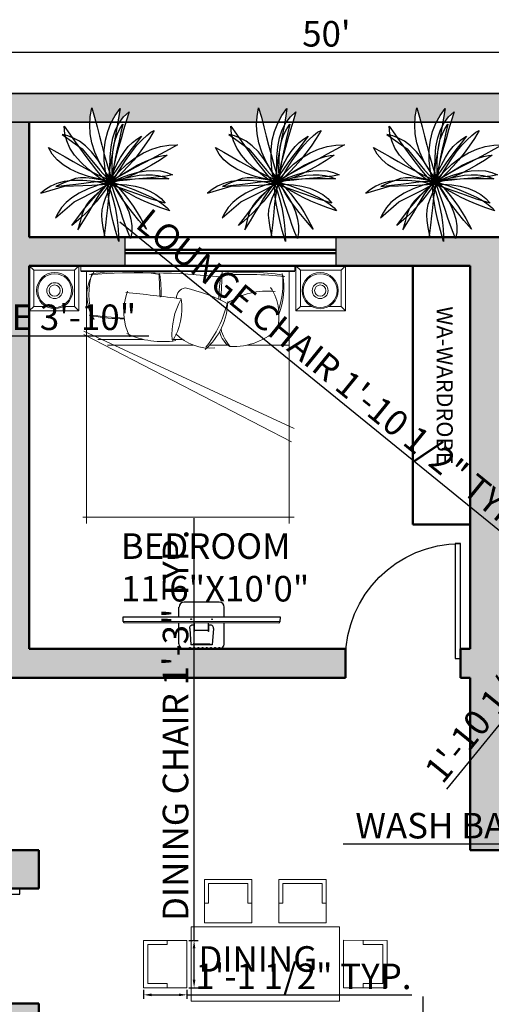
# Model space of a CAD drawing. Units: inches. Extents: x 2442 to 3851, y 589 to 2836.
# Tile 7 of 22: x 2698 to 2845, y 1717 to 2025. Entities that reach past the tile are written whole.
import ezdxf

# ---------------------------------------------------------------- set-up
doc = ezdxf.new("R2010")
doc.units = ezdxf.units.IN
for name, color, linetype, lineweight in [('0.10', 252, 'Continuous', 9), ('0.15', 34, 'Continuous', 15), ('A-ANNO-DIMS', 2, 'Continuous', 18), ('A-ANNO-TEXT', 7, 'Continuous', 18), ('A-AREA-IDEN', 7, 'Continuous', 18), ('A-DOOR', 4, 'Continuous', 25), ('A-FURN', 8, 'Continuous', 18), ('A-GLAZ', 1, 'Continuous', 25), ('A-WALL', 7, 'Continuous', 50), ('A-WALL-PATT', 8, 'Continuous', 13), ('C-PROP', 7, 'Continuous', 35), ('L-PLNT', 94, 'Continuous', 18)]:
    doc.layers.add(name, color=color, linetype=linetype, lineweight=lineweight)
doc.layers.add('DIENHOA', color=3, linetype='Continuous')
doc.layers.add('window', color=130, linetype='Continuous')
doc.styles.get("Standard").update_dxf_attribs({"font": 'arial.ttf'})
doc.dimstyles.new('ISO-25', dxfattribs={"dimtxt": 8, "dimasz": 2.5, "dimexe": 1.25, "dimexo": 0.625, "dimtad": 1, "dimlunit": 3, "dimtxsty": 'Standard', "dimcen": 2.5, "dimadec": 0, "dimazin": 0, "dimtfac": 1, "dimtmove": 0, "dimatfit": 3, "dimfxl": 1, "dimarcsym": 0})

# ---------------------------------------------------------------- blocks, each defined once
blk = doc.blocks.new('*U23')
for p, q in [((0, 0), (0, -6)), ((36, 0), (36, -6))]:
    blk.add_line(p, q)
blk.add_lwpolyline([(0, 0), (0, 36), (1.75, 36), (1.75, 0)], close=True)
blk.add_arc((0, 0), 36, 0, 90)
blk = doc.blocks.new('camita')
at = {"layer": '0.10'}
for p, q in [((-0.85, -0.045), (0.85, -0.045)), ((-0.805, -0.045), (-0.805, -2.0485)), ((0.805, -0.045), (0.805, -2.0485)), ((-0.8271, -0.521), (0.8464, -1.2932)), ((-0.8271, -0.5476), (0.8236, -1.3992)), ((-0.7161, -0.585), (-0.3554, -0.585)), ((-0.1136, -0.585), (-0.0485, -0.585)), ((-0.638, -0.63), (0.0434, -0.63)), ((0.1749, -0.63), (0.3179, -0.63)), ((0.4739, -0.63), (0.805, -0.63)), ((-0.8354, -2), (0.8464, -2))]:
    blk.add_line(p, q, dxfattribs=at)
blk.add_lwpolyline([(-0.85, -0.0405), (0.85, -0.0405), (0.85, 0), (-0.85, 0)], close=True, dxfattribs=at)
for centre, radius, start, end in [((-0.4574, -0.2364), 0.3443, 147.50996, 213.83359), ((-0.1997, -0.2266), 0.5864, 163.92635, 197.14087), ((-0.3639, -5.8457), 5.7909, 83.80731, 94.12107), ((-0.5104, -1.7232), 1.6781, 80.12554, 98.66187), ((2.3534, -0.0532), 2.5803, 180.10628, 184.38541), ((-1.5443, -0.2452), 1.3333, 359.93941, 7.55329), ((1.5815, -0.2893), 1.3353, 170.38021, 178.99138), ((-1.4396, -0.0609), 1.7117, 352.92911, 0.39592), ((0.4524, -3.0675), 2.9996, 83.90257, 93.67595), ((0.4863, -1.6286), 1.5781, 80.16015, 98.05996), ((0.0294, -0.1377), 0.7262, 342.58415, 6.00484), ((0.1326, -0.1696), 0.6307, 339.92303, 8.74334), ((-0.0543, -0.3633), 0.4542, 159.30257, 206.50263), ((-1.3301, -9.6748), 9.4985, 82.27078, 84.93989), ((-0.007, -0.258), 0.0828, 100.01798, 179.73597), ((-0.2931, -1.4378), 1.2903, 61.97485, 77.84351), ((0.6265, -0.7518), 0.5508, 82.96906, 124.67388), ((0.3203, -0.3944), 0.4043, 341.45245, 33.45121), ((0.4585, -0.5454), 0.5842, 151.04555, 184.14969), ((-0.5341, -0.3393), 0.4875, 327.26442, 9.0473), ((-0.1986, -0.2742), 0.5159, 310.73945, 359.05759), ((-0.5673, -0.0868), 0.9057, 321.69527, 346.46261), ((-1.8672, -14.986), 14.6323, 84.65974, 85.75157), ((-0.4598, 1.4861), 1.9092, 260.95299, 268.65169), ((-0.2002, 0.064), 0.6673, 244.78094, 279.06058), ((0.179, -0.272), 0.3828, 224.52836, 275.22287), ((0.4384, -0.4834), 0.1898, 193.68485, 236.70352), ((0.5707, -0.4317), 0.3145, 192.93877, 221.96363), ((0.3612, -0.133), 0.5096, 267.25889, 315.29965)]:
    blk.add_arc(centre, radius, start, end, dxfattribs=at)
blk = doc.blocks.new('VELADOR')
at = {"layer": '0.15'}
for p, q in [((-0.2475, 0), (-0.2025, -0.045)), ((0.2475, 0), (0.2025, -0.045)), ((-0.2025, -0.405), (-0.2475, -0.45)), ((0.2475, -0.45), (0.2025, -0.405))]:
    blk.add_line(p, q, dxfattribs=at)
blk.add_lwpolyline([(-0.2475, 0), (-0.2475, -0.45), (0.2475, -0.45), (0.2475, 0)], close=True, dxfattribs=at)
blk.add_lwpolyline([(0.0921, -0.405), (0.2025, -0.405), (0.2025, -0.045), (-0.2025, -0.045), (-0.2025, -0.405), (-0.0818, -0.405)], dxfattribs=at)
for radius in [0.18, 0.1688, 0.0788, 0.0563]:
    blk.add_circle((0.0052, -0.2474), radius, dxfattribs=at)
blk = doc.blocks.new('TV')
at = {"color": 0}
for p, q in [((3967.27, 1784.85), (3967.05, 1784.65)), ((3967.76, 1763.68), (3967.54, 1763.86))]:
    blk.add_line(p, q, dxfattribs=at)
at = {"layer": 'window'}
for p, q in [((3967.54, 1763.86), (3967.05, 1784.65)), ((3964.41, 1777.23), (3967.22, 1777.3)), ((3968.01, 1777.32), (3969.36, 1777.35)), ((3966.53, 1775.82), (3964.33, 1775.61)), ((3964.34, 1775.34), (3964.45, 1775.34)), ((3964.34, 1775.31), (3964.43, 1775.32)), ((3966.14, 1775.2), (3967.01, 1775.22)), ((3966.14, 1775.18), (3967.27, 1775.2)), ((3966.14, 1775.18), (3966.14, 1775.2)), ((3966.3, 1773.29), (3966.26, 1775.18)), ((3964.39, 1773.06), (3964.48, 1773.06)), ((3964.39, 1773.04), (3964.5, 1773.04)), ((3966.61, 1772.66), (3964.4, 1772.77)), ((3966.19, 1773.28), (3967.31, 1773.31)), ((3966.19, 1773.26), (3967.05, 1773.28)), ((3966.19, 1773.26), (3966.19, 1773.28)), ((3964.55, 1771.15), (3967.36, 1771.22)), ((3968.15, 1771.24), (3969.5, 1771.27))]:
    blk.add_line(p, q, dxfattribs=at)
for points in [[(3968.33, 1763.69), (3967.83, 1784.86), (3967.27, 1784.85), (3967.76, 1763.68), (3968.33, 1763.69)], [(3963.86, 1771.81), (3963.75, 1776.54)], [(3964.4, 1772.77), (3964.33, 1775.61)], [(3970.16, 1771.96), (3970.05, 1776.69)], [(3964.48, 1773.06), (3964.43, 1775.32)], [(3964.5, 1773.04), (3964.45, 1775.34)]]:
    blk.add_lwpolyline(points, dxfattribs=at)
for points in [[(3966.53, 1775.82, -0.263666), (3966.93, 1775.69), (3967, 1775.57), (3967.01, 1775.22)], [(3966.61, 1772.66, 0.263666), (3967, 1772.81), (3967.06, 1772.93), (3967.05, 1773.28)]]:
    blk.add_lwpolyline(points, format="xyb", dxfattribs=at)
for centre, radius in [((3963.91, 1775.73), 0.0679), ((3967.77, 1775.68), 0.0451), ((3963.93, 1775.17), 0.0679), ((3963.94, 1774.6), 0.0679), ((3963.95, 1774.04), 0.0679), ((3963.97, 1773.48), 0.0679), ((3963.98, 1772.92), 0.0679), ((3967.83, 1772.86), 0.0451), ((3963.99, 1772.35), 0.0679), ((3964.01, 1771.79), 0.0679)]:
    blk.add_circle(centre, radius, dxfattribs=at)
for centre, start, end in [((3964.42, 1776.56), 91.3414, 181.3414), ((3969.38, 1776.67), 1.3414, 91.3414), ((3964.53, 1771.83), 181.3414, 271.3414), ((3969.49, 1771.94), 271.3414, 1.3414)]:
    blk.add_arc(centre, 0.676, start, end, dxfattribs=at)
blk = doc.blocks.new('Cay03_mb')
at = {"layer": 'DIENHOA'}
for p, q in [((118.6, 555.3), (166.2, 599.1)), ((166.2, 599.1), (142.2, 519.4)), ((79.5, 503.7), (118.6, 555.3)), ((142.2, 519.4), (119, 441.7)), ((25.5, 374.3), (48.6, 443.6)), ((48.6, 443.6), (79.5, 503.7)), ((119, 441.7), (96.7, 365.6)), ((-365.2, 390.3), (-414.4, 402.8)), ((-414.4, 402.8), (-240.2, 277.8)), ((-314.9, 371.3), (-365.2, 390.3)), ((-263.5, 343.5), (-314.9, 371.3)), ((-211.2, 304.6), (-263.5, 343.5)), ((9.9, 295.3), (25.5, 374.3)), ((96.7, 365.6), (75.6, 290.6)), ((-240.2, 277.8), (-88.4, 94.9)), ((-158, 252.3), (-211.2, 304.6)), ((1.6, 205.7), (9.9, 295.3)), ((75.6, 290.6), (55.7, 216.3)), ((290.6, 243.2), (363.4, 275.4)), ((363.4, 275.4), (436.8, 297.2)), ((436.8, 297.2), (511, 309.6)), ((511.8, 271.4), (437.6, 231.5)), ((511, 309.6), (585.9, 313.5)), ((585.9, 313.5), (511.8, 271.4)), ((-104.2, 184.4), (-158, 252.3)), ((-49.6, 98.5), (-104.2, 184.4)), ((0.2, 104.9), (1.6, 205.7)), ((55.7, 216.3), (37.3, 142.1)), ((147, 144.1), (218.5, 199.8)), ((218.5, 199.8), (290.6, 243.2)), ((363.7, 192.9), (290.2, 154.9)), ((437.6, 231.5), (363.7, 192.9)), ((-88.4, 94.9), (5.4, -7.8)), ((5.4, -7.8), (-49.6, 98.5)), ((5.4, -7.8), (0.2, 104.9)), ((37.3, 142.1), (20.5, 67.6)), ((75.9, 75.2), (147, 144.1)), ((217.4, 116.6), (145.5, 77.3)), ((290.2, 154.9), (217.4, 116.6)), ((-345, 5.4), (-399.6, -17.1)), ((-298.6, 20.1), (-345, 5.4)), ((-254.7, 27.4), (-298.6, 20.1)), ((-208, 27.8), (-254.7, 27.4)), ((-152.7, 21.7), (-208, 27.8)), ((-83.4, 9.7), (-152.7, 21.7)), ((5.4, -7.8), (-83.4, 9.7)), ((5.4, -7.8), (75.9, 75.2)), ((20.5, 67.6), (5.4, -7.8)), ((74.7, 36.1), (5.4, -7.8)), ((5.4, -7.8), (100.3, 18.4)), ((46.3, 0.9), (5.4, -7.8)), ((96.7, 7.5), (46.3, 0.9)), ((145.5, 77.3), (74.7, 36.1)), ((155, 12.2), (96.7, 7.5)), ((100.3, 18.4), (182.2, 37.2)), ((219.6, 15.4), (155, 12.2)), ((182.2, 37.2), (253, 48.9)), ((289, 17.4), (219.6, 15.4)), ((253, 48.9), (314.6, 54.1)), ((361.6, 18.5), (289, 17.4)), ((314.6, 54.1), (369.2, 53.3)), ((435.8, 18.9), (361.6, 18.5)), ((369.2, 53.3), (418.6, 46.8)), ((418.6, 46.8), (464.9, 35.2)), ((510, 19), (435.8, 18.9)), ((464.9, 35.2), (510, 19)), ((-399.6, -17.1), (-468, -47.9)), ((-468, -47.9), (-375.6, -37.8)), ((-375.6, -37.8), (-295.3, -27.9)), ((-295.3, -27.9), (-225.8, -18.9)), ((-225.8, -18.9), (-165.8, -11.3)), ((-165.8, -11.3), (-114, -5.7)), ((-120.2, -122.1), (-79.8, -79.6)), ((-114, -5.7), (-69, -2.9)), ((-79.8, -79.6), (-45.1, -46.3)), ((-33.2, -69.5), (-74.6, -127.3)), ((-69, -2.9), (-29.6, -3.4)), ((-45.1, -46.3), (-16.5, -22.4)), ((5.4, -7.8), (-33.2, -69.5)), ((-29.6, -3.4), (5.4, -7.8)), ((-16.5, -22.4), (5.4, -7.8)), ((5.4, -7.8), (56.8, -73.3)), ((25.9, -64.4), (5.4, -7.8)), ((5.4, -7.8), (112.8, -40.3)), ((53.5, -41.6), (5.4, -7.8)), ((47, -125.9), (25.9, -64.4)), ((107, -75.7), (53.5, -41.6)), ((56.8, -73.3), (100.4, -139.1)), ((165.5, -109.6), (107, -75.7)), ((112.8, -40.3), (207.5, -73.8)), ((207.5, -73.8), (289.5, -107.6)), ((-165.9, -174.1), (-120.2, -122.1)), ((-74.6, -127.3), (-117.8, -181.1)), ((68.7, -190.6), (47, -125.9)), ((100.4, -139.1), (135.9, -204.3)), ((228.7, -142.8), (165.5, -109.6)), ((296, -174.7), (228.7, -142.8)), ((289.5, -107.6), (359.3, -141.1)), ((359.3, -141.1), (416.9, -173.5)), ((-271, -306.6), (-216.3, -235.6)), ((-216.3, -235.6), (-165.9, -174.1)), ((-162.1, -230.9), (-206.3, -276.5)), ((-117.8, -181.1), (-162.1, -230.9)), ((90.8, -256.6), (68.7, -190.6)), ((135.9, -204.3), (162.8, -268.3)), ((367.1, -204.8), (296, -174.7)), ((441.6, -232.7), (367.1, -204.8)), ((416.9, -173.5), (462.6, -204.2)), ((518.9, -257.7), (441.6, -232.7)), ((462.6, -204.2), (496.5, -232.5)), ((496.5, -232.5), (518.9, -257.7)), ((-329.5, -387.1), (-271, -306.6)), ((-249.6, -317.8), (-291, -354.7)), ((-206.3, -276.5), (-249.6, -317.8)), ((113.1, -322.2), (90.8, -256.6)), ((135.4, -385.6), (113.1, -322.2)), ((162.8, -268.3), (181, -330.4)), ((181, -330.4), (190, -390)), ((-291, -354.7), (-329.5, -387.1)), ((157.6, -445), (135.4, -385.6)), ((190, -390), (189.6, -446.3)), ((179.5, -498.7), (157.6, -445)), ((189.6, -446.3), (179.5, -498.7))]:
    blk.add_line(p, q, dxfattribs=at)
for points in [[(23.7, -5.4), (-41, 82.2), (-91.8, 167.1), (-129.7, 249.5), (-155.6, 329.6), (-170.2, 407.8), (-174.7, 484.2), (-169.8, 559.3), (-156.5, 633.1)], [(-156.5, 633.1), (-132.5, 551.3), (-110.5, 470), (-89.8, 389.2), (-69.6, 309), (-49, 229.4), (-27.1, 150.4), (-3.2, 72.1), (23.7, -5.4)], [(-16.4, -26.7), (-38.3, 80), (-48.9, 178.3), (-48.7, 269), (-38.5, 352.6), (-19.1, 429.7), (9, 501), (44.9, 567.1), (87.9, 628.5)], [(87.9, 628.5), (75.5, 544.2), (61.3, 461.2), (46.1, 379.1), (30.8, 297.8), (16.1, 216.9), (2.9, 136), (-8.3, 54.9), (-16.4, -26.7)], [(-395.6, 473.7), (-347.5, 405.6), (-300.6, 339.5), (-254.3, 275.1), (-208.3, 212.3), (-161.9, 150.9), (-114.8, 90.7), (-66.5, 31.6), (-16.4, -26.7)], [(-16.4, -26.7), (-108.3, 38.6), (-186.9, 101.7), (-252.4, 163.5), (-305.1, 224.4), (-345.4, 285.2), (-373.7, 346.6), (-390.4, 409.2), (-395.6, 473.7)], [(23.7, -5.4), (19.8, 93), (20.3, 177), (25, 248.5), (34, 309.8), (47.3, 362.7), (64.9, 409.3), (86.8, 451.7), (112.9, 491.9)], [(112.9, 491.9), (96, 419.7), (79.5, 347.4), (63.9, 276.5), (50, 208.4), (38.4, 144.8), (29.7, 86.9), (24.6, 36.3), (23.7, -5.4)], [(384.3, 437.5), (342.2, 367.8), (298.1, 301.7), (252.6, 239.4), (206.1, 181.1), (159.4, 127.2), (113, 78), (67.6, 33.6), (23.7, -5.4)], [(23.7, -5.4), (79.9, 91.7), (134.1, 176.2), (185.8, 248.4), (234.3, 308.7), (279, 357.3), (319.3, 394.8), (354.6, 421.4), (384.3, 437.5)], [(273.2, 387.3), (227.6, 328.8), (182.3, 270.1), (138.4, 212.3), (97.2, 156.4), (60, 103.4), (27.8, 54.6), (1.9, 10.8), (-16.4, -26.7)], [(-16.4, -26.7), (21.4, 64.2), (57, 140.3), (91.4, 203.3), (125.2, 255.1), (159.5, 297.5), (195, 332.5), (232.7, 361.8), (273.2, 387.3)], [(-530.5, 289.7), (-458.3, 248.1), (-387.9, 207.8), (-318.9, 168.7), (-250.8, 131.1), (-182.9, 94.8), (-114.9, 59.9), (-46.2, 26.5), (23.7, -5.4)], [(23.7, -5.4), (-87.2, 15.2), (-185, 39.6), (-270.3, 68.2), (-343.7, 101.4), (-405.9, 139.7), (-457.3, 183.5), (-498.7, 233.4), (-530.5, 289.7)], [(496.7, 224), (429.4, 178.4), (361.6, 136.9), (294.1, 99.5), (227.5, 66.1), (162.4, 36.7), (99.7, 11.5), (39.8, -9.7), (-16.4, -26.7)], [(-16.4, -26.7), (75.4, 37.9), (160.1, 91.8), (237.3, 135.7), (306.6, 170), (367.6, 195.4), (419.9, 212.5), (463.1, 221.9), (496.7, 224)], [(23.7, -5.4), (99.3, 29.7), (173.2, 57.1), (244.8, 76.7), (313.3, 88.3), (377.9, 91.8), (437.9, 87), (492.7, 73.8), (541.4, 52)], [(-16.4, -26.7), (-134, -4.7), (-235.3, 5.3), (-322, 4.7), (-395.9, -5), (-458.7, -22.3), (-512.3, -45.7), (-558.2, -73.6), (-598.4, -104.7)], [(541.4, 52), (484.1, 42.9), (421.2, 34.8), (354.4, 27.6), (285.4, 20.9), (216.1, 14.5), (148.2, 8.1), (83.5, 1.6), (23.7, -5.4)], [(-598.4, -104.7), (-392.7, -44.4), (-155, -37.4), (-16.4, -26.7)], [(-471.9, -320.3), (-310.5, -179.3), (-97.7, -73.3), (23.7, -5.4)], [(23.7, -5.4), (-92.3, -34.8), (-188.4, -68.2), (-266.9, -105.1), (-329.9, -144.9), (-379.7, -187), (-418.5, -230.7), (-448.5, -275.3), (-471.9, -320.3)], [(-276.2, -424.4), (-227.3, -345.4), (-185.7, -276.1), (-150, -215.7), (-119.1, -163.8), (-91.5, -119.5), (-66, -82.3), (-41.4, -51.6), (-16.4, -26.7)], [(-16.4, -26.7), (-84.9, -86), (-137, -133.1), (-175.8, -173), (-204.3, -210), (-225.5, -249.1), (-242.5, -294.7), (-258.4, -351.6), (-276.2, -424.4)], [(23.7, -5.4), (-13.6, -87.9), (-41.1, -152.6), (-59.6, -205), (-69.9, -250.7), (-72.8, -295), (-69.2, -343.6), (-59.7, -401.9), (-45.3, -475.5)], [(-45.3, -475.5), (-34.1, -383.2), (-25.4, -302.8), (-18.3, -233.1), (-12, -172.9), (-5.6, -121.2), (2, -76.8), (11.4, -38.5), (23.7, -5.4)], [(76.2, -524.2), (48.8, -428.5), (26.6, -341.7), (9.2, -264.1), (-3.6, -196.1), (-12.3, -138), (-17.1, -90.2), (-18.3, -53), (-16.4, -26.7)], [(-16.4, -26.7), (66.9, -26.6), (145.6, -32.7), (218.8, -44.9), (285.8, -63.1), (345.9, -87.1), (398.4, -116.6), (442.6, -151.6), (477.6, -191.8)], [(477.6, -191.8), (421.8, -176), (361.3, -156.9), (297.6, -135.5), (232.2, -112.6), (166.6, -89.4), (102.3, -66.6), (40.8, -45.4), (-16.4, -26.7)], [(-16.4, -26.7), (8.5, -95.1), (28.5, -163.3), (44.3, -230.6), (56.3, -296.1), (65, -359), (70.9, -418.5), (74.5, -473.9), (76.2, -524.2)], [(316.5, -418.1), (251.4, -342.8), (194.8, -273.3), (146.5, -210.2), (106.3, -153.8), (74.1, -104.7), (49.7, -63.4), (32.9, -30.1), (23.7, -5.4)], [(23.7, -5.4), (74.9, -57.1), (121.8, -110.6), (164.3, -165), (202.7, -219.4), (237, -272.9), (267.3, -324.5), (293.7, -373.2), (316.5, -418.1)]]:
    blk.add_lwpolyline(points, dxfattribs=at)
blk = doc.blocks.new('*D31')
at = {"layer": 'A-ANNO-DIMS', "color": 0, "lineweight": -2, "transparency": 16777216}
for p, q in [((2493.6, 2002.49), (2493.6, 2016.02)), ((2496.1, 2014.77), (3091.1, 2014.77)), ((3093.6, 2002.49), (3093.6, 2016.02))]:
    blk.add_line(p, q, dxfattribs=at)
at = {"layer": 'A-ANNO-DIMS', "color": 0, "transparency": 16777216}
for points in [[(2496.1, 2015.19), (2496.1, 2014.36), (2493.6, 2014.77)], [(3091.1, 2015.19), (3091.1, 2014.36), (3093.6, 2014.77)]]:
    blk.add_solid(points, dxfattribs=at)
at = {"layer": 'Defpoints', "color": 0, "transparency": 16777216}
for p in [(3093.6, 2014.77), (2493.6, 2001.86), (3093.6, 2001.86)]:
    blk.add_point(p, dxfattribs=at)
at = {"layer": 'A-ANNO-DIMS', "color": 0, "transparency": 16777216, "insert": (2793.6, 2019.48), "char_height": 8, "attachment_point": 5}
blk.add_mtext("50'", dxfattribs=at)
blk = doc.blocks.new('CHAIR-DINING')
for p, q in [((0, 14.84), (13.57, 14.84)), ((0, 0), (0, 14.84)), ((1.28, 13.56), (7.42, 13.56)), ((1.28, 1.32), (1.28, 13.56)), ((7.42, 13.56), (7.42, 14.84)), ((13.57, 0), (13.57, 14.84)), ((0, 0), (13.57, 0)), ((7.42, 1.32), (1.28, 1.32)), ((7.42, 0), (7.42, 1.32))]:
    blk.add_line(p, q)
blk = doc.blocks.new('*D144')
at = {"layer": 'A-ANNO-DIMS', "color": 0, "lineweight": -2, "transparency": 16777216}
for p, q in [((2857.1, 1857.27), (2728.92, 1961.48)), ((2858.85, 1859.43), (2856.31, 1856.3)), ((2872.8, 1844.49), (2859.04, 1855.69)), ((2876.5, 1845.08), (2873.96, 1841.94))]:
    blk.add_line(p, q, dxfattribs=at)
at = {"layer": 'A-ANNO-DIMS', "color": 0, "transparency": 16777216}
for points in [[(2859.3, 1856.01), (2858.77, 1855.36), (2857.1, 1857.27)], [(2873.07, 1844.82), (2872.54, 1844.17), (2874.74, 1842.91)]]:
    blk.add_solid(points, dxfattribs=at)
at = {"layer": 'Defpoints', "color": 0, "transparency": 16777216}
for p in [(2859.25, 1859.91), (2857.1, 1857.27), (2876.9, 1845.56)]:
    blk.add_point(p, dxfattribs=at)
at = {"layer": 'A-ANNO-DIMS', "color": 0, "transparency": 16777216, "insert": (2795.04, 1913.86), "char_height": 8, "attachment_point": 5, "rotation": 320.8857}
blk.add_mtext('LOUNGE CHAIR 1\'-10 1/2" TYP.', dxfattribs=at)
blk = doc.blocks.new('*D145')
at = {"layer": 'A-ANNO-DIMS', "color": 0, "lineweight": -2, "transparency": 16777216}
for p, q in [((2891.54, 1862.58), (2894.67, 1860.03)), ((2892.13, 1858.88), (2881.12, 1845.35)), ((2877.38, 1845.17), (2880.51, 1842.62)), ((2879.54, 1843.41), (2831.21, 1783.96))]:
    blk.add_line(p, q, dxfattribs=at)
at = {"layer": 'A-ANNO-DIMS', "color": 0, "transparency": 16777216}
for points in [[(2891.8, 1859.15), (2892.45, 1858.62), (2893.7, 1860.82)], [(2880.8, 1845.61), (2881.45, 1845.09), (2879.54, 1843.41)]]:
    blk.add_solid(points, dxfattribs=at)
at = {"layer": 'Defpoints', "color": 0, "transparency": 16777216}
for p in [(2891.06, 1862.98), (2876.9, 1845.56), (2879.54, 1843.41)]:
    blk.add_point(p, dxfattribs=at)
at = {"layer": 'A-ANNO-DIMS', "color": 0, "transparency": 16777216, "insert": (2850.89, 1815.72), "char_height": 8, "attachment_point": 5, "rotation": 50.8857}
blk.add_mtext('1\'-10 1/2" TYP.', dxfattribs=at)
blk = doc.blocks.new('*D148')
at = {"layer": 'A-ANNO-DIMS', "color": 0, "lineweight": -2, "transparency": 16777216}
for p, q in [((2752.18, 1736.61), (2752.18, 1868.82)), ((2750.58, 1736.61), (2753.43, 1736.61)), ((2752.18, 1724.27), (2752.18, 1734.11)), ((2750.58, 1721.77), (2753.43, 1721.77))]:
    blk.add_line(p, q, dxfattribs=at)
at = {"layer": 'A-ANNO-DIMS', "color": 0, "transparency": 16777216}
for points in [[(2751.76, 1734.11), (2752.59, 1734.11), (2752.18, 1736.61)], [(2751.76, 1724.27), (2752.59, 1724.27), (2752.18, 1721.77)]]:
    blk.add_solid(points, dxfattribs=at)
at = {"layer": 'Defpoints', "color": 0, "transparency": 16777216}
for p in [(2749.95, 1736.61), (2752.18, 1736.61), (2749.95, 1721.77)]:
    blk.add_point(p, dxfattribs=at)
at = {"layer": 'A-ANNO-DIMS', "color": 0, "transparency": 16777216, "insert": (2747.41, 1803.97), "char_height": 8, "attachment_point": 5, "rotation": 90}
blk.add_mtext('DINING CHAIR 1\'-3" TYP.', dxfattribs=at)
blk = doc.blocks.new('*D149')
at = {"layer": 'A-ANNO-DIMS', "color": 0, "lineweight": -2, "transparency": 16777216}
for p, q in [((2736.38, 1721.15), (2736.38, 1718.3)), ((2749.95, 1721.15), (2749.95, 1718.3)), ((2738.88, 1719.55), (2747.45, 1719.55)), ((2749.95, 1719.55), (2820.35, 1719.55))]:
    blk.add_line(p, q, dxfattribs=at)
at = {"layer": 'A-ANNO-DIMS', "color": 0, "transparency": 16777216}
for points in [[(2738.88, 1719.96), (2738.88, 1719.13), (2736.38, 1719.55)], [(2747.45, 1719.96), (2747.45, 1719.13), (2749.95, 1719.55)]]:
    blk.add_solid(points, dxfattribs=at)
at = {"layer": 'Defpoints', "color": 0, "transparency": 16777216}
for p in [(2736.38, 1721.77), (2749.95, 1721.77), (2749.95, 1719.55)]:
    blk.add_point(p, dxfattribs=at)
at = {"layer": 'A-ANNO-DIMS', "color": 0, "transparency": 16777216, "insert": (2786.4, 1724.31), "char_height": 8, "attachment_point": 5}
blk.add_mtext('1\'-1 1/2" TYP.', dxfattribs=at)
blk = doc.blocks.new('*D154')
at = {"layer": 'A-ANNO-DIMS', "color": 0, "lineweight": -2, "transparency": 16777216}
for p, q in [((2765.6, 1687.48), (2641.71, 1687.48)), ((2765.6, 1684.49), (2765.6, 1688.73)), ((2787.22, 1687.48), (2768.1, 1687.48)), ((2789.72, 1684.49), (2789.72, 1688.73))]:
    blk.add_line(p, q, dxfattribs=at)
at = {"layer": 'A-ANNO-DIMS', "color": 0, "transparency": 16777216}
for points in [[(2768.1, 1687.9), (2768.1, 1687.07), (2765.6, 1687.48)], [(2787.22, 1687.9), (2787.22, 1687.07), (2789.72, 1687.48)]]:
    blk.add_solid(points, dxfattribs=at)
at = {"layer": 'Defpoints', "color": 0, "transparency": 16777216}
for p in [(2765.6, 1687.48), (2765.6, 1683.86), (2789.72, 1683.86)]:
    blk.add_point(p, dxfattribs=at)
at = {"layer": 'A-ANNO-DIMS', "color": 0, "transparency": 16777216, "insert": (2702.4, 1692.25), "char_height": 8, "attachment_point": 5}
blk.add_mtext('SOFA CHAIR 2\'-0" TYP.', dxfattribs=at)
blk = doc.blocks.new('*D158')
at = {"layer": 'A-ANNO-DIMS', "color": 0, "lineweight": -2, "transparency": 16777216}
for p, q in [((2943.6, 1765.49), (2943.6, 1767.98)), ((2956.06, 1765.49), (2956.06, 1767.98)), ((2943.6, 1766.73), (2798.84, 1766.73)), ((2953.56, 1766.73), (2946.1, 1766.73))]:
    blk.add_line(p, q, dxfattribs=at)
at = {"layer": 'A-ANNO-DIMS', "color": 0, "transparency": 16777216}
for points in [[(2946.1, 1767.15), (2946.1, 1766.32), (2943.6, 1766.73)], [(2953.56, 1767.15), (2953.56, 1766.32), (2956.06, 1766.73)]]:
    blk.add_solid(points, dxfattribs=at)
at = {"layer": 'Defpoints', "color": 0, "transparency": 16777216}
for p in [(2943.6, 1766.73), (2943.6, 1764.86), (2956.06, 1764.86)]:
    blk.add_point(p, dxfattribs=at)
at = {"layer": 'A-ANNO-DIMS', "color": 0, "transparency": 16777216, "insert": (2869.97, 1771.49), "char_height": 8, "attachment_point": 5}
blk.add_mtext('WASH BASIN 1\'-0 1/2" TYP.', dxfattribs=at)
blk = doc.blocks.new('*D166')
at = {"layer": 'A-ANNO-DIMS', "color": 0, "lineweight": -2, "transparency": 16777216}
for p, q in [((2823.9, 1579.64), (2823.9, 1719)), ((2828.69, 1579.64), (2822.65, 1579.64)), ((2823.9, 1546), (2823.9, 1577.14)), ((2828.69, 1543.5), (2822.65, 1543.5))]:
    blk.add_line(p, q, dxfattribs=at)
at = {"layer": 'A-ANNO-DIMS', "color": 0, "transparency": 16777216}
for points in [[(2823.48, 1577.14), (2824.31, 1577.14), (2823.9, 1579.64)], [(2823.48, 1546), (2824.31, 1546), (2823.9, 1543.5)]]:
    blk.add_solid(points, dxfattribs=at)
at = {"layer": 'Defpoints', "color": 0, "transparency": 16777216}
for p in [(2823.9, 1579.64), (2829.32, 1579.64), (2829.32, 1543.5)]:
    blk.add_point(p, dxfattribs=at)
at = {"layer": 'A-ANNO-DIMS', "color": 0, "transparency": 16777216, "insert": (2819.13, 1650.57), "char_height": 8, "attachment_point": 5, "rotation": 90}
blk.add_mtext('COFFEE TABLE 3\'-0" TYP.', dxfattribs=at)
blk = doc.blocks.new('*D180')
at = {"layer": 'A-ANNO-DIMS', "color": 0, "lineweight": -2, "transparency": 16777216}
for p, q in [((2549.24, 1932.24), (2549.24, 1924.7)), ((2595.34, 1932.24), (2595.34, 1924.7)), ((2551.74, 1925.95), (2592.84, 1925.95)), ((2595.34, 1925.95), (2738.05, 1925.95))]:
    blk.add_line(p, q, dxfattribs=at)
at = {"layer": 'A-ANNO-DIMS', "color": 0, "transparency": 16777216}
for points in [[(2551.74, 1926.37), (2551.74, 1925.53), (2549.24, 1925.95)], [(2592.84, 1926.37), (2592.84, 1925.53), (2595.34, 1925.95)]]:
    blk.add_solid(points, dxfattribs=at)
at = {"layer": 'Defpoints', "color": 0, "transparency": 16777216}
for p in [(2549.24, 1932.86), (2595.34, 1932.86), (2595.34, 1925.95)]:
    blk.add_point(p, dxfattribs=at)
at = {"layer": 'A-ANNO-DIMS', "color": 0, "transparency": 16777216, "insert": (2667.94, 1930.71), "char_height": 8, "attachment_point": 5}
blk.add_mtext('WASHING MACHINE 3\'-10"', dxfattribs=at)

msp = doc.modelspace()

# ---------------------------------------------------------------- hatches: boundary and pattern name
at = {"layer": 'A-WALL-PATT'}
h = msp.add_hatch(color=256, dxfattribs=at)
h.dxf.hatch_style = 1
h.paths.add_polyline_path([(2502.599, 1992.864), (2719.571, 1992.864), (2719.687, 1994.649), (2720.167, 1997.319), (2721.479, 1992.864), (2726.325, 1992.864), (2727.448, 1994.93), (2729.005, 1997.153), (2728.372, 1992.864), (2728.871, 1992.864), (2730.114, 1994.505), (2731.833, 1996.09), (2730.966, 1993.206), (2730.864, 1992.864), (2771.772, 1992.864), (2771.887, 1994.649), (2772.368, 1997.319), (2773.68, 1992.864), (2778.526, 1992.864), (2779.649, 1994.93), (2781.206, 1997.153), (2780.572, 1992.864), (2781.072, 1992.864), (2782.315, 1994.505), (2784.034, 1996.09), (2783.167, 1993.206), (2783.065, 1992.864), (2821.282, 1992.864), (2821.398, 1994.649), (2821.878, 1997.319), (2823.19, 1992.864), (2828.036, 1992.864), (2829.159, 1994.93), (2830.716, 1997.153), (2830.083, 1992.864), (2830.582, 1992.864), (2831.825, 1994.505), (2833.544, 1996.09), (2832.677, 1993.206), (2832.575, 1992.864), (2869.287, 1992.864), (2869.403, 1994.649), (2869.884, 1997.319), (2871.195, 1992.864), (2876.042, 1992.864), (2877.165, 1994.93), (2878.721, 1997.153), (2878.088, 1992.864), (2878.587, 1992.864), (2879.83, 1994.505), (2881.55, 1996.09), (2880.682, 1993.206), (2880.58, 1992.864), (2919.335, 1992.864), (2919.451, 1994.649), (2919.932, 1997.319), (2921.243, 1992.864), (2926.09, 1992.864), (2927.213, 1994.93), (2928.77, 1997.153), (2928.136, 1992.864), (2928.635, 1992.864), (2929.878, 1994.505), (2931.598, 1996.09), (2930.73, 1993.206), (2930.628, 1992.864), (2966.155, 1992.864), (2966.27, 1994.649), (2966.751, 1997.319), (2968.063, 1992.864), (2972.909, 1992.864), (2974.032, 1994.93), (2975.589, 1997.153), (2974.955, 1992.864), (2975.455, 1992.864), (2976.698, 1994.505), (2978.417, 1996.09), (2977.55, 1993.206), (2977.448, 1992.864), (3010.53, 1992.864), (3010.646, 1994.649), (3011.127, 1997.319), (3012.438, 1992.864), (3017.285, 1992.864), (3018.408, 1994.93), (3019.964, 1997.153), (3019.331, 1992.864), (3019.83, 1992.864), (3021.073, 1994.505), (3022.793, 1996.09), (3021.925, 1993.206), (3021.823, 1992.864), (3057.996, 1992.864), (3058.45, 1995.382), (3059.191, 1992.864), (3065.64, 1992.864), (3067.287, 1995.216), (3066.94, 1992.864), (3068.717, 1992.864), (3070.116, 1994.153), (3069.728, 1992.864), (3084.599, 1992.864), (3084.599, 1983.791), (3085.291, 1983.828), (3084.599, 1983.434), (3084.599, 1932.114), (3085.291, 1932.151), (3084.599, 1931.757), (3084.599, 1886.278), (3085.291, 1886.315), (3084.599, 1885.921), (3084.599, 1410.864), (3066.599, 1410.864), (3066.599, 1401.864), (3093.599, 1401.864), (3093.599, 2001.864), (2493.599, 2001.864), (2493.599, 1401.864), (2538.599, 1401.864), (2538.599, 1410.864), (2502.599, 1410.864)])
h.paths.add_polyline_path([(2738.599, 1410.864), (2547.599, 1410.864), (2547.599, 1401.864), (2738.599, 1401.864)], flags=17)
h.paths.add_polyline_path([(2910.599, 1410.864), (2792.599, 1410.864), (2792.599, 1401.864), (2910.599, 1401.864), (2910.599, 1402.864)], flags=17)
h = msp.add_hatch(color=256, dxfattribs=at)
h.dxf.hatch_style = 1
h.paths.add_polyline_path([(2799.599, 1467.864), (2775.599, 1467.864), (2775.599, 1458.864), (2799.599, 1458.864)])
h.paths.add_polyline_path([(2703.599, 1506.864), (2670.599, 1506.864), (2670.599, 1497.864), (2694.599, 1497.864), (2694.599, 1458.864), (2733.599, 1458.864), (2733.599, 1467.864), (2709.417, 1467.864), (2703.599, 1467.864)])
h.paths.add_polyline_path([(2604.599, 1506.864), (2593.599, 1506.864), (2593.599, 1497.864), (2604.599, 1497.864)])
h.paths.add_polyline_path([(2547.599, 1497.864), (2553.599, 1497.864), (2553.599, 1506.864), (2547.599, 1506.864), (2547.599, 1530.864), (2538.599, 1530.864), (2538.599, 1401.864), (2547.599, 1401.864)])
h.paths.add_polyline_path([(2547.599, 1683.864), (2538.599, 1683.864), (2538.599, 1578.864), (2547.599, 1578.864), (2547.599, 1602.864), (2694.599, 1602.864), (2694.599, 1554.864), (2703.599, 1554.864), (2703.599, 1716.864), (2694.599, 1716.864), (2694.599, 1611.864), (2547.599, 1611.864)])
h.paths.add_polyline_path([(2892.599, 1497.864), (2883.599, 1497.864), (2883.599, 1488.228), (2883.599, 1467.864), (2865.599, 1467.864), (2865.599, 1458.864), (2892.599, 1458.864)])
h.paths.add_polyline_path([(3048.599, 1722.864), (3039.599, 1722.864), (3039.599, 1716.864), (2937.599, 1716.864), (2937.599, 1710.864), (3039.599, 1710.864), (3039.599, 1685.364), (3048.599, 1685.364)])
h.paths.add_polyline_path([(3048.599, 1779.864), (3039.599, 1779.864), (3039.599, 1773.864), (2961.599, 1773.864), (2961.599, 1791.864), (2955.599, 1791.864), (2955.599, 1773.864), (2895.599, 1773.864), (2895.599, 1821.864), (2916.599, 1821.864), (2916.599, 1827.864), (2889.599, 1827.864), (2889.599, 1773.864), (2886.599, 1773.864), (2886.599, 1764.864), (2937.599, 1764.864), (2937.599, 1746.864), (2943.599, 1746.864), (2943.599, 1764.864), (2956.06, 1764.864), (3039.599, 1764.864), (3039.599, 1758.864), (3048.599, 1758.864)])
h.paths.add_polyline_path([(3048.599, 1827.864), (2976.475, 1827.864, -0.1284593), (2975.705, 1827.665), (2964.694, 1827.687, -0.1198794), (2963.972, 1827.864), (2946.599, 1827.864), (2946.599, 1821.864), (3039.599, 1821.864), (3039.599, 1815.864), (3048.599, 1815.864)])
h.paths.add_polyline_path([(3048.599, 1956.864), (3023.366, 1956.864), (3023.277, 1956.402), (3023.088, 1956.864), (3019.494, 1956.864), (3019.543, 1955.479), (3019.146, 1956.864), (3015.599, 1956.864), (3015.599, 1947.864), (3039.599, 1947.864), (3039.599, 1875.864), (3048.599, 1875.864), (3048.599, 1880.743), (3047.576, 1881.614), (3046.081, 1883.417), (3044.931, 1885.453), (3047.541, 1883.949), (3048.599, 1883.343), (3048.599, 1910.588), (3047.049, 1909.235), (3047.896, 1910.862), (3048.599, 1911.909), (3048.599, 1918.826), (3042.477, 1917.032), (3043.928, 1918.154), (3045.59, 1919.165), (3047.525, 1920.009), (3048.599, 1920.305), (3048.599, 1926.579), (3047.576, 1927.45), (3046.081, 1929.252), (3044.931, 1931.289), (3047.541, 1929.785), (3048.599, 1929.179)])
h.paths.add_polyline_path([(2967.599, 1956.864), (2932.171, 1956.864), (2932.082, 1956.402), (2931.893, 1956.864), (2928.299, 1956.864), (2928.348, 1955.479), (2927.951, 1956.864), (2898.599, 1956.864), (2898.599, 1947.864), (2967.599, 1947.864)])
h.paths.add_polyline_path([(2850.599, 1956.864), (2834.118, 1956.864), (2834.029, 1956.402), (2833.84, 1956.864), (2830.245, 1956.864), (2830.294, 1955.479), (2829.897, 1956.864), (2796.599, 1956.864), (2796.599, 1947.864), (2799.599, 1947.864), (2838.599, 1947.864), (2838.599, 1827.864), (2835.599, 1827.864), (2835.599, 1824.864), (2835.599, 1818.864), (2838.599, 1818.864), (2838.599, 1764.864), (2850.599, 1764.864), (2850.599, 1770.864), (2850.599, 1773.864), (2847.599, 1773.864), (2847.599, 1947.864), (2850.599, 1947.864)])
h.paths.add_polyline_path([(2700.599, 1947.864), (2730.599, 1947.864), (2730.599, 1956.864), (2700.599, 1956.864), (2700.599, 1992.864), (2691.599, 1992.864), (2691.599, 1932.864), (2670.599, 1932.864), (2670.599, 1923.864), (2691.599, 1923.864), (2691.599, 1818.864), (2799.599, 1818.864), (2799.599, 1827.864), (2700.599, 1827.864)])
h.paths.add_polyline_path([(2640.599, 1932.864), (2538.599, 1932.864), (2538.599, 1868.364), (2547.599, 1868.364), (2547.599, 1923.864), (2640.599, 1923.864), (2640.599, 1929.864)])
h.paths.add_polyline_path([(2547.599, 1820.364), (2538.599, 1820.364), (2538.599, 1731.864), (2547.599, 1731.864), (2547.599, 1755.864), (2694.599, 1755.864), (2694.599, 1752.864), (2697.599, 1752.864), (2703.599, 1752.864), (2703.599, 1764.864), (2547.599, 1764.864)])
h.paths.add_polyline_path([(2725.858, 1838.187), (2790.115, 1838.187), (2790.115, 1868.602), (2725.858, 1868.602)], flags=25)
h.paths.add_polyline_path([(2892.599, 1671.864), (2883.599, 1671.864), (2883.599, 1563.864), (2892.599, 1563.864), (2892.599, 1602.864), (3048.599, 1602.864), (3048.599, 1637.364), (3039.599, 1637.364), (3039.599, 1611.864), (2892.599, 1611.864)])

# ---------------------------------------------------------------- linework, layer by layer
at = {"layer": 'A-FURN'}
for p, q in [((2751.228, 1740.841), (2797.705, 1740.841)), ((2751.228, 1717.579), (2751.228, 1740.841)), ((2797.705, 1740.841), (2797.705, 1717.579)), ((2797.705, 1717.579), (2751.228, 1717.579))]:
    msp.add_line(p, q, dxfattribs=at)
at = {"layer": 'A-GLAZ'}
for p, q in [((2730.599, 1947.864), (2730.599, 1956.864)), ((2796.599, 1947.864), (2796.599, 1956.864))]:
    msp.add_line(p, q, dxfattribs=at)
at = {"layer": 'A-WALL'}
for p, q in [((2700.599, 1956.864), (2700.599, 1992.864)), ((2700.599, 1956.864), (3048.599, 1956.864)), ((2730.599, 1952.864), (2796.599, 1952.864)), ((2730.599, 1951.864), (2796.599, 1951.864)), ((2700.599, 1947.864), (2838.599, 1947.864)), ((2700.599, 1827.864), (2700.599, 1947.864)), ((2820.599, 1866.864), (2820.599, 1947.864)), ((2838.599, 1827.864), (2838.599, 1947.864)), ((2820.599, 1866.864), (2838.599, 1866.864)), ((2700.599, 1827.864), (2799.599, 1827.864)), ((2799.599, 1818.864), (2799.599, 1827.864)), ((2835.599, 1818.864), (2835.599, 1827.864)), ((2835.599, 1827.864), (2838.599, 1827.864)), ((2691.599, 1818.864), (2799.599, 1818.864)), ((2835.599, 1818.864), (2838.599, 1818.864)), ((2838.599, 1764.864), (2838.599, 1818.864)), ((2547.599, 1764.864), (2703.599, 1764.864)), ((2703.599, 1752.864), (2703.599, 1764.864)), ((2838.599, 1764.864), (2850.599, 1764.864)), ((2694.599, 1752.864), (2703.599, 1752.864)), ((2694.599, 1716.864), (2703.599, 1716.864)), ((2703.599, 1554.864), (2703.599, 1716.864))]:
    msp.add_line(p, q, dxfattribs=at)
at = {"layer": 'C-PROP'}
for points in [[(3066.599, 1401.864), (3093.599, 1401.864), (3093.599, 2001.864), (2493.599, 2001.864), (2493.599, 1401.864), (2738.599, 1401.864)], [(3066.599, 1410.864), (3084.599, 1410.864), (3084.599, 1992.864), (2502.599, 1992.864), (2502.599, 1410.864), (2538.599, 1410.864)]]:
    msp.add_lwpolyline(points, dxfattribs=at)

# ---------------------------------------------------------------- block references
at = {"layer": 'A-DOOR', "xscale": -1}
msp.add_blockref('*U23', (2835.599, 1824.864), dxfattribs=at)
at = {"layer": 'A-DOOR', "xscale": -1, "rotation": 90}
msp.add_blockref('*U23', (2697.599, 1752.864), dxfattribs=at)
at = {"layer": 'A-FURN'}
for name, p, xscale, yscale, zscale in [('VELADOR', (2708.374, 1947.864), 31.41542173157097, 31.41542173157097, 31.41542173157097), ('camita', (2750.205, 1947.864), 39.375, 39.375, 39.375)]:
    msp.add_blockref(name, p, dxfattribs=dict(at, xscale=xscale, yscale=yscale, zscale=zscale))
for name, p, xscale, yscale, zscale, rotation in [('VELADOR', (2791.823, 1947.864), -31.41542173157097, 31.41542173157097, 31.41542173157097, 359.9999999999999), ('TV', (6647.703, -7499.166), 2.327319231123021, 2.327319231123021, 2.327319231123021, 88.54308451816127)]:
    msp.add_blockref(name, p, dxfattribs=dict(at, xscale=xscale, yscale=yscale, zscale=zscale, rotation=rotation))
for p, rotation in [((2755.424, 1755.681), 269.9293303373234), ((2778.668, 1755.674), 269.9790238270802), ((2812.562, 1736.62), 179.9314884092627)]:
    msp.add_blockref('CHAIR-DINING', p, dxfattribs=dict(at, rotation=rotation))
msp.add_blockref('CHAIR-DINING', (2736.383, 1721.771), dxfattribs=at)
at = {"layer": 'L-PLNT', "xscale": 0.036152509973097, "yscale": 0.036152509973097, "zscale": 0.036152509973097}
for p in [(2725.827, 1974.43), (2778.028, 1974.43), (2827.538, 1974.43)]:
    msp.add_blockref('Cay03_mb', p, dxfattribs=at)

# ---------------------------------------------------------------- texts
at = {"layer": 'A-ANNO-TEXT', "insert": (2833.144, 1935.167), "char_height": 5, "attachment_point": 1, "rotation": 270}
msp.add_mtext_dynamic_manual_height_columns('{\\fTimes New Roman|b0|i0|c0|p18;WA-WARDROBE}', width=110.76054, gutter_width=12.5, heights=[0], dxfattribs=at)
at = {"layer": 'A-AREA-IDEN', "char_height": 8, "attachment_point": 1}
for s, insert in [('{\\fTimes New Roman|b0|i0|c0|p18;BEDROOM\\P11\'6"X10\'0"}', (2729.242, 1864.076)), ('{\\fTimes New Roman|b0|i0|c0|p18;DINING}', (2753.513, 1734.785))]:
    msp.add_mtext_dynamic_manual_height_columns(s, width=110.76054, gutter_width=12.5, heights=[0], dxfattribs=dict(at, insert=insert))

# ---------------------------------------------------------------- dimensions: what is measured, and where the dimension line sits
at = {"layer": 'A-ANNO-DIMS'}
dim = msp.add_linear_dim(base=(3093.599, 2014.775), p1=(2493.599, 2001.864), p2=(3093.599, 2001.864), dimstyle='ISO-25', override={"dimclrd": 0, "dimclre": 0, "dimclrt": 0}, dxfattribs=at)
dim.commit()
dim.dimension.update_dxf_attribs({"geometry": '*D31', "text_midpoint": (2793.599, 2019.485)})
for base, p1, p2, angle, text, picture, middle in [((2857.095, 1857.265), (2876.897, 1845.562), (2859.248, 1859.913), 140.88565, 'LOUNGE CHAIR <> TYP.', '*D144', (2795.044, 1913.859)), ((2752.176, 1736.609), (2749.951, 1721.771), (2749.951, 1736.609), 90, 'DINING CHAIR <> TYP.', '*D148', (2747.412, 1803.966)), ((2879.545, 1843.409), (2891.056, 1862.976), (2876.897, 1845.562), 230.88565, '<> TYP.', '*D145', (2850.894, 1815.72)), ((2943.599, 1766.733), (2956.06, 1764.864), (2943.599, 1764.864), 180, 'WASH BASIN <> TYP.', '*D158', (2869.969, 1771.495)), ((2765.598, 1687.482), (2789.72, 1683.864), (2765.598, 1683.864), 180, 'SOFA CHAIR <> TYP.', '*D154', (2702.404, 1692.247)), ((2823.898, 1579.637), (2829.318, 1543.504), (2829.318, 1579.637), 90, 'COFFEE TABLE <> TYP.', '*D166', (2819.131, 1650.568))]:
    dim = msp.add_linear_dim(base=base, p1=p1, p2=p2, angle=angle, text=text, dimstyle='ISO-25', override={"dimdec": 1, "dimrnd": 0, "dimzin": 1, "dimlunit": 4, "dimfrac": 2}, dxfattribs=at)
    dim.commit()
    dim.dimension.update_dxf_attribs({"geometry": picture, "text_midpoint": middle})
for base, p1, p2, text, picture, middle in [((2595.344, 1925.949), (2549.243, 1932.864), (2595.344, 1932.864), 'WASHING MACHINE <>', '*D180', (2667.945, 1930.713)), ((2749.951, 1719.546), (2736.383, 1721.771), (2749.951, 1721.771), '<> TYP.', '*D149', (2786.402, 1724.307))]:
    dim = msp.add_linear_dim(base=base, p1=p1, p2=p2, text=text, dimstyle='ISO-25', override={"dimdec": 1, "dimrnd": 0, "dimzin": 1, "dimlunit": 4, "dimfrac": 2}, dxfattribs=at)
    dim.commit()
    dim.dimension.update_dxf_attribs({"geometry": picture, "text_midpoint": middle})

doc.saveas('drawing.dxf')
